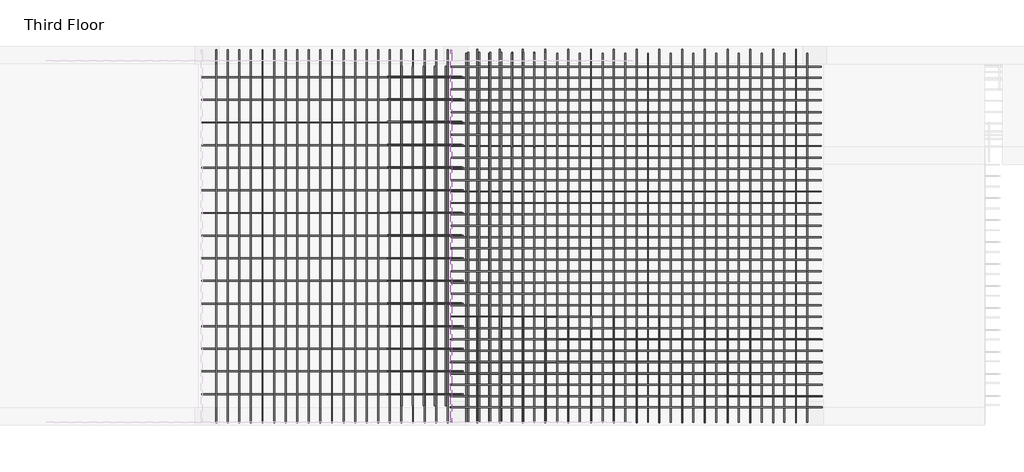
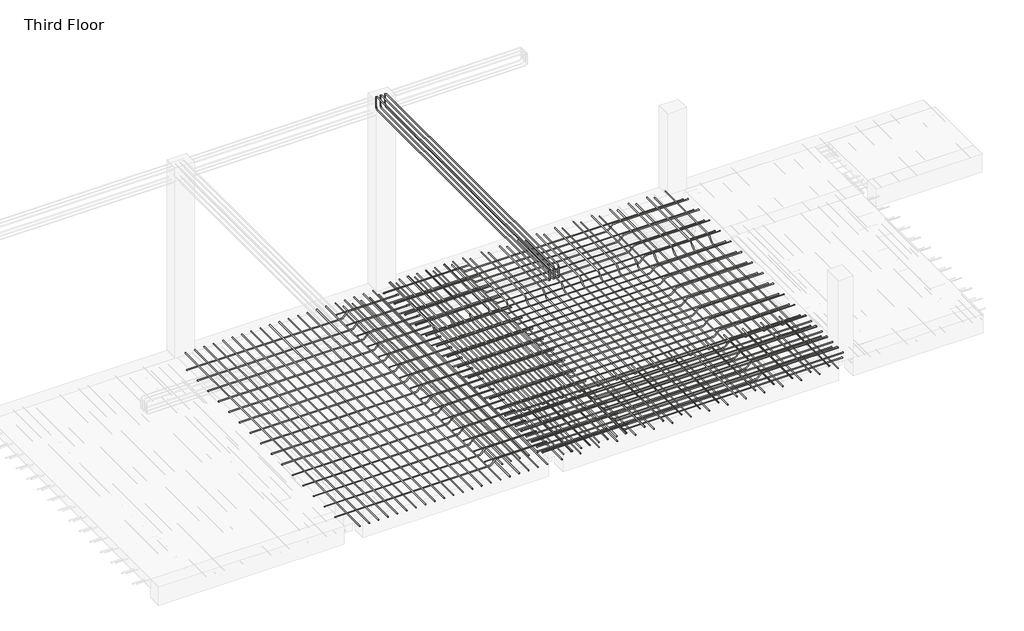
# One storey, part 3 of 4: 14 reinforcing bars.
"""IFC4 building model written with IfcOpenShell, lengths in millimetres."""

from ifc_helpers import new_model, si_unit, point, frame, origin, place, context, project, spatial, polyline, circle_curve, trimmed, segment, composite_curve, source, transform, mapped, element, save
from ifc_brep_helpers import swept_disk

model = new_model("IFC4")

# Units and contexts
model_context = context("Model", 3, world=origin())
ifc_project = project(units=[si_unit("LENGTHUNIT", "METRE", prefix="MILLI")], contexts=[model_context])

# Site, building, storey
site = spatial("IfcSite", under=ifc_project)
building = spatial("IfcBuilding", under=site)
storey = spatial("IfcBuildingStorey", under=building, Name="Third Floor", Elevation=9601.2)

# Reinforcing bars
placement = place(None, origin())
reinforcing_bar_shape = source(origin(), model_context, "Body", "SolidModel", [
    swept_disk(composite_curve([segment(polyline([(-2909.6112474, 5017.2334631, 12564.4994949), (-2909.6112474, 5017.2334631, 12712.4994949)]), True, "CONTINUOUS"), segment(trimmed(circle_curve(frame((-2909.6112474, 4971.2334631, 12712.4994949), z_axis=(1.0, 0.0, 0.0), x_axis=(0.0, 46.0, 0.0)), 46.0), [point((-2909.6112474, 5017.2334631, 12712.4994949))], [point((-2909.6112474, 4971.2334631, 12758.4994949))], True, "CARTESIAN"), True, "CONTINUOUS"), segment(polyline([(-2909.6112474, 4971.2334631, 12758.4994949), (-2909.6112474, 278.4334631, 12758.4994949)]), True, "CONTINUOUS"), segment(trimmed(circle_curve(frame((-2909.6112474, 278.4334631, 12712.4994949), z_axis=(1.0, 0.0, 0.0), x_axis=(0.0, 0.0, 46.0)), 46.0), [point((-2909.6112474, 278.4334631, 12758.4994949))], [point((-2909.6112474, 232.4334631, 12712.4994949))], True, "CARTESIAN"), True, "CONTINUOUS"), segment(polyline([(-2909.6112474, 232.4334631, 12712.4994949), (-2909.6112474, 232.4334631, 12564.4994949)]), True, "CONTINUOUS")], self_intersect=False), 6.0),
])
element("IfcReinforcingBar", 1, at=placement, inside=storey, context=model_context, shape_type="MappedRepresentation", body=[
    mapped(reinforcing_bar_shape, transform((0.0, 0.0, 0.0), x_axis=(1.0, 0.0, 0.0), y_axis=(0.0, 1.0, 0.0), z_axis=(0.0, 0.0, 1.0))),
    mapped(reinforcing_bar_shape, transform((71.1994949, 0.0, 0.0), x_axis=(1.0, 0.0, 0.0), y_axis=(0.0, 1.0, 0.0), z_axis=(0.0, 0.0, 1.0))),
    mapped(reinforcing_bar_shape, transform((142.3989899, 0.0, 0.0), x_axis=(1.0, 0.0, 0.0), y_axis=(0.0, 1.0, 0.0), z_axis=(0.0, 0.0, 1.0))),
])
reinforcing_bar_2_shape = source(origin(), model_context, "Body", "SolidModel", [
    swept_disk(composite_curve([segment(polyline([(-2909.6112474, 5017.2334631, 12733.9005051), (-2909.6112474, 5017.2334631, 12585.9005051)]), True, "CONTINUOUS"), segment(trimmed(circle_curve(frame((-2909.6112474, 4971.2334631, 12585.9005051), z_axis=(-1.0, 0.0, 0.0), x_axis=(0.0, 46.0, 0.0)), 46.0), [point((-2909.6112474, 5017.2334631, 12585.9005051))], [point((-2909.6112474, 4971.2334631, 12539.9005051))], True, "CARTESIAN"), True, "CONTINUOUS"), segment(polyline([(-2909.6112474, 4971.2334631, 12539.9005051), (-2909.6112474, 278.4334631, 12539.9005051)]), True, "CONTINUOUS"), segment(trimmed(circle_curve(frame((-2909.6112474, 278.4334631, 12585.9005051), z_axis=(-1.0, 0.0, 0.0), x_axis=(0.0, 0.0, -46.0)), 46.0), [point((-2909.6112474, 278.4334631, 12539.9005051))], [point((-2909.6112474, 232.4334631, 12585.9005051))], True, "CARTESIAN"), True, "CONTINUOUS"), segment(polyline([(-2909.6112474, 232.4334631, 12585.9005051), (-2909.6112474, 232.4334631, 12733.9005051)]), True, "CONTINUOUS")], self_intersect=False), 6.0),
])
element("IfcReinforcingBar", 2, at=placement, inside=storey, context=model_context, shape_type="MappedRepresentation", body=[
    mapped(reinforcing_bar_2_shape, transform((0.0, 0.0, 0.0), x_axis=(1.0, 0.0, 0.0), y_axis=(0.0, 1.0, 0.0), z_axis=(0.0, 0.0, 1.0))),
    mapped(reinforcing_bar_2_shape, transform((71.1994949, 0.0, 0.0), x_axis=(1.0, 0.0, 0.0), y_axis=(0.0, 1.0, 0.0), z_axis=(0.0, 0.0, 1.0))),
    mapped(reinforcing_bar_2_shape, transform((142.3989899, 0.0, 0.0), x_axis=(1.0, 0.0, 0.0), y_axis=(0.0, 1.0, 0.0), z_axis=(0.0, 0.0, 1.0))),
])
reinforcing_bar_3_shape = source(origin(), model_context, "Body", "SolidModel", [
    swept_disk(composite_curve([segment(polyline([(-2755.5109354, 590.4513536, 9570.2), (-3537.444222, 590.4513536, 9570.2)]), True, "CONTINUOUS"), segment(trimmed(circle_curve(frame((-3537.444222, 590.4513536, 9524.2), z_axis=(0.0, -1.0, 0.0), x_axis=(0.0, 0.0, 46.0)), 46.0), [point((-3537.444222, 590.4513536, 9570.2))], [point((-3569.9711339, 590.4513536, 9556.7269119))], True, "CARTESIAN"), True, "CONTINUOUS"), segment(polyline([(-3569.9711339, 590.4513536, 9556.7269119), (-3633.4249578, 590.4513536, 9493.2730881)]), True, "CONTINUOUS"), segment(trimmed(circle_curve(frame((-3665.9518697, 590.4513536, 9525.8), z_axis=(0.0, 1.0000000000000002, 0.0), x_axis=(32.52691189999996, 0.0, -32.526911899998595)), 46.0), [point((-3633.4249578, 590.4513536, 9493.2730881))], [point((-3665.9518697, 590.4513536, 9479.8))], True, "CARTESIAN"), True, "CONTINUOUS"), segment(polyline([(-3665.9518697, 590.4513536, 9479.8), (-6120.96376, 590.4513536, 9479.8)]), True, "CONTINUOUS")], self_intersect=False), 6.0),
])
element("IfcReinforcingBar", 3, at=placement, inside=storey, context=model_context, shape_type="MappedRepresentation", body=[
    mapped(reinforcing_bar_3_shape, transform((0.0, 0.0, 0.0), x_axis=(1.0, 0.0, 0.0), y_axis=(0.0, 1.0, 0.0), z_axis=(0.0, 0.0, 1.0))),
    mapped(reinforcing_bar_3_shape, transform((0.0, 291.2629007, 0.0), x_axis=(1.0, 0.0, 0.0), y_axis=(0.0, 1.0, 0.0), z_axis=(0.0, 0.0, 1.0))),
    mapped(reinforcing_bar_3_shape, transform((0.0, 582.5258014, 0.0), x_axis=(1.0, 0.0, 0.0), y_axis=(0.0, 1.0, 0.0), z_axis=(0.0, 0.0, 1.0))),
    mapped(reinforcing_bar_3_shape, transform((0.0, 873.7887021, 0.0), x_axis=(1.0, 0.0, 0.0), y_axis=(0.0, 1.0, 0.0), z_axis=(0.0, 0.0, 1.0))),
    mapped(reinforcing_bar_3_shape, transform((0.0, 1165.0516028, 0.0), x_axis=(1.0, 0.0, 0.0), y_axis=(0.0, 1.0, 0.0), z_axis=(0.0, 0.0, 1.0))),
    mapped(reinforcing_bar_3_shape, transform((0.0, 1456.3145035, 0.0), x_axis=(1.0, 0.0, 0.0), y_axis=(0.0, 1.0, 0.0), z_axis=(0.0, 0.0, 1.0))),
    mapped(reinforcing_bar_3_shape, transform((0.0, 1747.5774042, 0.0), x_axis=(1.0, 0.0, 0.0), y_axis=(0.0, 1.0, 0.0), z_axis=(0.0, 0.0, 1.0))),
    mapped(reinforcing_bar_3_shape, transform((0.0, 2038.8403049, 0.0), x_axis=(1.0, 0.0, 0.0), y_axis=(0.0, 1.0, 0.0), z_axis=(0.0, 0.0, 1.0))),
    mapped(reinforcing_bar_3_shape, transform((0.0, 2330.1032056, 0.0), x_axis=(1.0, 0.0, 0.0), y_axis=(0.0, 1.0, 0.0), z_axis=(0.0, 0.0, 1.0))),
    mapped(reinforcing_bar_3_shape, transform((0.0, 2621.3661063, 0.0), x_axis=(1.0, 0.0, 0.0), y_axis=(0.0, 1.0, 0.0), z_axis=(0.0, 0.0, 1.0))),
    mapped(reinforcing_bar_3_shape, transform((0.0, 2912.629007, 0.0), x_axis=(1.0, 0.0, 0.0), y_axis=(0.0, 1.0, 0.0), z_axis=(0.0, 0.0, 1.0))),
    mapped(reinforcing_bar_3_shape, transform((0.0, 3203.8919077, 0.0), x_axis=(1.0, 0.0, 0.0), y_axis=(0.0, 1.0, 0.0), z_axis=(0.0, 0.0, 1.0))),
    mapped(reinforcing_bar_3_shape, transform((0.0, 3495.1548084, 0.0), x_axis=(1.0, 0.0, 0.0), y_axis=(0.0, 1.0, 0.0), z_axis=(0.0, 0.0, 1.0))),
    mapped(reinforcing_bar_3_shape, transform((0.0, 3786.4177091, 0.0), x_axis=(1.0, 0.0, 0.0), y_axis=(0.0, 1.0, 0.0), z_axis=(0.0, 0.0, 1.0))),
    mapped(reinforcing_bar_3_shape, transform((0.0, 4077.6806098, 0.0), x_axis=(1.0, 0.0, 0.0), y_axis=(0.0, 1.0, 0.0), z_axis=(0.0, 0.0, 1.0))),
])
reinforcing_bar_4_shape = source(origin(), model_context, "Body", "SolidModel", [
    swept_disk(composite_curve([segment(polyline([(-3546.4250876, 4809.6334631, 9559.9006995), (-3546.4250876, 440.0334631, 9559.9006995)]), True, "CONTINUOUS")], self_intersect=False), 6.0),
])
element("IfcReinforcingBar", 4, at=placement, inside=storey, context=model_context, shape_type="MappedRepresentation", body=[
    mapped(reinforcing_bar_4_shape, transform((0.0, 0.0, 0.0), x_axis=(1.0, 0.0, 0.0), y_axis=(0.0, 1.0, 0.0), z_axis=(0.0, 0.0, 1.0))),
    mapped(reinforcing_bar_4_shape, transform((140.6783338, 0.0, 0.0), x_axis=(1.0, 0.0, 0.0), y_axis=(0.0, 1.0, 0.0), z_axis=(0.0, 0.0, 1.0))),
    mapped(reinforcing_bar_4_shape, transform((281.3566676, 0.0, 0.0), x_axis=(1.0, 0.0, 0.0), y_axis=(0.0, 1.0, 0.0), z_axis=(0.0, 0.0, 1.0))),
    mapped(reinforcing_bar_4_shape, transform((422.0350014, 0.0, 0.0), x_axis=(1.0, 0.0, 0.0), y_axis=(0.0, 1.0, 0.0), z_axis=(0.0, 0.0, 1.0))),
    mapped(reinforcing_bar_4_shape, transform((562.7133352, 0.0, 0.0), x_axis=(1.0, 0.0, 0.0), y_axis=(0.0, 1.0, 0.0), z_axis=(0.0, 0.0, 1.0))),
])
reinforcing_bar_5_shape = source(origin(), model_context, "Body", "SolidModel", [
    swept_disk(composite_curve([segment(polyline([(-2778.2123639, 4678.4115375, 9572.2), (-3737.2865297, 4678.4115375, 9572.2)]), True, "CONTINUOUS")], self_intersect=False), 4.0),
])
element("IfcReinforcingBar", 5, at=placement, inside=storey, context=model_context, shape_type="MappedRepresentation", body=[
    mapped(reinforcing_bar_5_shape, transform((0.0, 0.0, 0.0), x_axis=(1.0, 0.0, 0.0), y_axis=(0.0, 1.0, 0.0), z_axis=(0.0, 0.0, 1.0))),
    mapped(reinforcing_bar_5_shape, transform((0.0, -291.8025106, 0.0), x_axis=(1.0, 0.0, 0.0), y_axis=(0.0, 1.0, 0.0), z_axis=(0.0, 0.0, 1.0))),
    mapped(reinforcing_bar_5_shape, transform((0.0, -583.6050212, 0.0), x_axis=(1.0, 0.0, 0.0), y_axis=(0.0, 1.0, 0.0), z_axis=(0.0, 0.0, 1.0))),
    mapped(reinforcing_bar_5_shape, transform((0.0, -875.4075319, 0.0), x_axis=(1.0, 0.0, 0.0), y_axis=(0.0, 1.0, 0.0), z_axis=(0.0, 0.0, 1.0))),
    mapped(reinforcing_bar_5_shape, transform((0.0, -1167.2100425, 0.0), x_axis=(1.0, 0.0, 0.0), y_axis=(0.0, 1.0, 0.0), z_axis=(0.0, 0.0, 1.0))),
    mapped(reinforcing_bar_5_shape, transform((0.0, -1459.0125531, 0.0), x_axis=(1.0, 0.0, 0.0), y_axis=(0.0, 1.0, 0.0), z_axis=(0.0, 0.0, 1.0))),
    mapped(reinforcing_bar_5_shape, transform((0.0, -1750.8150637, 0.0), x_axis=(1.0, 0.0, 0.0), y_axis=(0.0, 1.0, 0.0), z_axis=(0.0, 0.0, 1.0))),
    mapped(reinforcing_bar_5_shape, transform((0.0, -2042.6175743, 0.0), x_axis=(1.0, 0.0, 0.0), y_axis=(0.0, 1.0, 0.0), z_axis=(0.0, 0.0, 1.0))),
    mapped(reinforcing_bar_5_shape, transform((0.0, -2334.420085, 0.0), x_axis=(1.0, 0.0, 0.0), y_axis=(0.0, 1.0, 0.0), z_axis=(0.0, 0.0, 1.0))),
    mapped(reinforcing_bar_5_shape, transform((0.0, -2626.2225956, 0.0), x_axis=(1.0, 0.0, 0.0), y_axis=(0.0, 1.0, 0.0), z_axis=(0.0, 0.0, 1.0))),
    mapped(reinforcing_bar_5_shape, transform((0.0, -2918.0251062, 0.0), x_axis=(1.0, 0.0, 0.0), y_axis=(0.0, 1.0, 0.0), z_axis=(0.0, 0.0, 1.0))),
    mapped(reinforcing_bar_5_shape, transform((0.0, -3209.8276168, 0.0), x_axis=(1.0, 0.0, 0.0), y_axis=(0.0, 1.0, 0.0), z_axis=(0.0, 0.0, 1.0))),
    mapped(reinforcing_bar_5_shape, transform((0.0, -3501.6301274, 0.0), x_axis=(1.0, 0.0, 0.0), y_axis=(0.0, 1.0, 0.0), z_axis=(0.0, 0.0, 1.0))),
    mapped(reinforcing_bar_5_shape, transform((0.0, -3793.4326381, 0.0), x_axis=(1.0, 0.0, 0.0), y_axis=(0.0, 1.0, 0.0), z_axis=(0.0, 0.0, 1.0))),
    mapped(reinforcing_bar_5_shape, transform((0.0, -4085.2351487, 0.0), x_axis=(1.0, 0.0, 0.0), y_axis=(0.0, 1.0, 0.0), z_axis=(0.0, 0.0, 1.0))),
])
reinforcing_bar_6_shape = source(origin(), model_context, "Body", "SolidModel", [
    swept_disk(composite_curve([segment(polyline([(-2956.7117524, 218.9117605, 9488.3387401), (-2956.7117524, 5019.9992064, 9488.3387401)]), True, "CONTINUOUS")], self_intersect=False), 6.0),
])
element("IfcReinforcingBar", 6, at=placement, inside=storey, context=model_context, shape_type="MappedRepresentation", body=[
    mapped(reinforcing_bar_6_shape, transform((0.0, 0.0, 0.0), x_axis=(1.0, 0.0, 0.0), y_axis=(0.0, 1.0, 0.0), z_axis=(0.0, 0.0, 1.0))),
    mapped(reinforcing_bar_6_shape, transform((-149.025, 0.0, 0.0), x_axis=(1.0, 0.0, 0.0), y_axis=(0.0, 1.0, 0.0), z_axis=(0.0, 0.0, 1.0))),
    mapped(reinforcing_bar_6_shape, transform((-298.05, 0.0, 0.0), x_axis=(1.0, 0.0, 0.0), y_axis=(0.0, 1.0, 0.0), z_axis=(0.0, 0.0, 1.0))),
    mapped(reinforcing_bar_6_shape, transform((-447.075, 0.0, 0.0), x_axis=(1.0, 0.0, 0.0), y_axis=(0.0, 1.0, 0.0), z_axis=(0.0, 0.0, 1.0))),
    mapped(reinforcing_bar_6_shape, transform((-596.1, 0.0, 0.0), x_axis=(1.0, 0.0, 0.0), y_axis=(0.0, 1.0, 0.0), z_axis=(0.0, 0.0, 1.0))),
    mapped(reinforcing_bar_6_shape, transform((-745.125, 0.0, 0.0), x_axis=(1.0, 0.0, 0.0), y_axis=(0.0, 1.0, 0.0), z_axis=(0.0, 0.0, 1.0))),
    mapped(reinforcing_bar_6_shape, transform((-894.15, 0.0, 0.0), x_axis=(1.0, 0.0, 0.0), y_axis=(0.0, 1.0, 0.0), z_axis=(0.0, 0.0, 1.0))),
    mapped(reinforcing_bar_6_shape, transform((-1043.175, 0.0, 0.0), x_axis=(1.0, 0.0, 0.0), y_axis=(0.0, 1.0, 0.0), z_axis=(0.0, 0.0, 1.0))),
    mapped(reinforcing_bar_6_shape, transform((-1192.2, 0.0, 0.0), x_axis=(1.0, 0.0, 0.0), y_axis=(0.0, 1.0, 0.0), z_axis=(0.0, 0.0, 1.0))),
    mapped(reinforcing_bar_6_shape, transform((-1341.225, 0.0, 0.0), x_axis=(1.0, 0.0, 0.0), y_axis=(0.0, 1.0, 0.0), z_axis=(0.0, 0.0, 1.0))),
    mapped(reinforcing_bar_6_shape, transform((-1490.25, 0.0, 0.0), x_axis=(1.0, 0.0, 0.0), y_axis=(0.0, 1.0, 0.0), z_axis=(0.0, 0.0, 1.0))),
    mapped(reinforcing_bar_6_shape, transform((-1639.275, 0.0, 0.0), x_axis=(1.0, 0.0, 0.0), y_axis=(0.0, 1.0, 0.0), z_axis=(0.0, 0.0, 1.0))),
    mapped(reinforcing_bar_6_shape, transform((-1788.3, 0.0, 0.0), x_axis=(1.0, 0.0, 0.0), y_axis=(0.0, 1.0, 0.0), z_axis=(0.0, 0.0, 1.0))),
    mapped(reinforcing_bar_6_shape, transform((-1937.325, 0.0, 0.0), x_axis=(1.0, 0.0, 0.0), y_axis=(0.0, 1.0, 0.0), z_axis=(0.0, 0.0, 1.0))),
    mapped(reinforcing_bar_6_shape, transform((-2086.35, 0.0, 0.0), x_axis=(1.0, 0.0, 0.0), y_axis=(0.0, 1.0, 0.0), z_axis=(0.0, 0.0, 1.0))),
    mapped(reinforcing_bar_6_shape, transform((-2235.375, 0.0, 0.0), x_axis=(1.0, 0.0, 0.0), y_axis=(0.0, 1.0, 0.0), z_axis=(0.0, 0.0, 1.0))),
    mapped(reinforcing_bar_6_shape, transform((-2384.4, 0.0, 0.0), x_axis=(1.0, 0.0, 0.0), y_axis=(0.0, 1.0, 0.0), z_axis=(0.0, 0.0, 1.0))),
    mapped(reinforcing_bar_6_shape, transform((-2533.425, 0.0, 0.0), x_axis=(1.0, 0.0, 0.0), y_axis=(0.0, 1.0, 0.0), z_axis=(0.0, 0.0, 1.0))),
    mapped(reinforcing_bar_6_shape, transform((-2682.45, 0.0, 0.0), x_axis=(1.0, 0.0, 0.0), y_axis=(0.0, 1.0, 0.0), z_axis=(0.0, 0.0, 1.0))),
    mapped(reinforcing_bar_6_shape, transform((-2831.475, 0.0, 0.0), x_axis=(1.0, 0.0, 0.0), y_axis=(0.0, 1.0, 0.0), z_axis=(0.0, 0.0, 1.0))),
    mapped(reinforcing_bar_6_shape, transform((-2980.5, 0.0, 0.0), x_axis=(1.0, 0.0, 0.0), y_axis=(0.0, 1.0, 0.0), z_axis=(0.0, 0.0, 1.0))),
])
reinforcing_bar_7_shape = source(origin(), model_context, "Body", "SolidModel", [
    swept_disk(composite_curve([segment(polyline([(-1702.6950858, 4992.3164819, 9554.9006995), (-1702.6950858, 234.3272052, 9554.9006995)]), True, "CONTINUOUS")], self_intersect=False), 6.0),
])
element("IfcReinforcingBar", 7, at=placement, inside=storey, context=model_context, shape_type="MappedRepresentation", body=[
    mapped(reinforcing_bar_7_shape, transform((0.0, 0.0, 0.0), x_axis=(1.0, 0.0, 0.0), y_axis=(0.0, 1.0, 0.0), z_axis=(0.0, 0.0, 1.0))),
    mapped(reinforcing_bar_7_shape, transform((-141.4880952, 0.0, 0.0), x_axis=(1.0, 0.0, 0.0), y_axis=(0.0, 1.0, 0.0), z_axis=(0.0, 0.0, 1.0))),
    mapped(reinforcing_bar_7_shape, transform((-282.9761905, 0.0, 0.0), x_axis=(1.0, 0.0, 0.0), y_axis=(0.0, 1.0, 0.0), z_axis=(0.0, 0.0, 1.0))),
    mapped(reinforcing_bar_7_shape, transform((-424.4642857, 0.0, 0.0), x_axis=(1.0, 0.0, 0.0), y_axis=(0.0, 1.0, 0.0), z_axis=(0.0, 0.0, 1.0))),
    mapped(reinforcing_bar_7_shape, transform((-565.952381, 0.0, 0.0), x_axis=(1.0, 0.0, 0.0), y_axis=(0.0, 1.0, 0.0), z_axis=(0.0, 0.0, 1.0))),
    mapped(reinforcing_bar_7_shape, transform((-707.4404762, 0.0, 0.0), x_axis=(1.0, 0.0, 0.0), y_axis=(0.0, 1.0, 0.0), z_axis=(0.0, 0.0, 1.0))),
    mapped(reinforcing_bar_7_shape, transform((-848.9285714, 0.0, 0.0), x_axis=(1.0, 0.0, 0.0), y_axis=(0.0, 1.0, 0.0), z_axis=(0.0, 0.0, 1.0))),
    mapped(reinforcing_bar_7_shape, transform((-990.4166667, 0.0, 0.0), x_axis=(1.0, 0.0, 0.0), y_axis=(0.0, 1.0, 0.0), z_axis=(0.0, 0.0, 1.0))),
])
reinforcing_bar_8_shape = source(origin(), model_context, "Body", "SolidModel", [
    swept_disk(composite_curve([segment(polyline([(-2905.905155, 4803.6334631, 9567.1687876), (-1727.9771661, 4803.6334631, 9567.1687876)]), True, "CONTINUOUS"), segment(trimmed(circle_curve(frame((-1727.9771661, 4803.6334631, 9521.1687876), z_axis=(0.0, 1.0, 0.0), x_axis=(0.0, 0.0, 46.0)), 46.0), [point((-1727.9771661, 4803.6334631, 9567.1687876))], [point((-1695.4502541, 4803.6334631, 9553.6956996))], True, "CARTESIAN"), True, "CONTINUOUS"), segment(polyline([(-1695.4502541, 4803.6334631, 9553.6956996), (-1634.9899166, 4803.6334631, 9493.2353621)]), True, "CONTINUOUS"), segment(trimmed(circle_curve(frame((-1602.4630047, 4803.6334631, 9525.762274), z_axis=(0.0, -1.0, 0.0), x_axis=(-32.52691189999996, 0.0, -32.526911900000414)), 46.0), [point((-1634.9899166, 4803.6334631, 9493.2353621))], [point((-1602.4630047, 4803.6334631, 9479.762274))], True, "CARTESIAN"), True, "CONTINUOUS"), segment(polyline([(-1602.4630047, 4803.6334631, 9479.762274), (1847.5013288, 4803.6334631, 9479.762274)]), True, "CONTINUOUS")], self_intersect=False), 6.0),
])
element("IfcReinforcingBar", 8, at=placement, inside=storey, context=model_context, shape_type="MappedRepresentation", body=[
    mapped(reinforcing_bar_8_shape, transform((0.0, 0.0, 0.0), x_axis=(1.0, 0.0, 0.0), y_axis=(0.0, 1.0, 0.0), z_axis=(0.0, 0.0, 1.0))),
    mapped(reinforcing_bar_8_shape, transform((0.0, -292.3066667, 0.0), x_axis=(1.0, 0.0, 0.0), y_axis=(0.0, 1.0, 0.0), z_axis=(0.0, 0.0, 1.0))),
    mapped(reinforcing_bar_8_shape, transform((0.0, -584.6133333, 0.0), x_axis=(1.0, 0.0, 0.0), y_axis=(0.0, 1.0, 0.0), z_axis=(0.0, 0.0, 1.0))),
    mapped(reinforcing_bar_8_shape, transform((0.0, -876.92, 0.0), x_axis=(1.0, 0.0, 0.0), y_axis=(0.0, 1.0, 0.0), z_axis=(0.0, 0.0, 1.0))),
    mapped(reinforcing_bar_8_shape, transform((0.0, -1169.2266667, 0.0), x_axis=(1.0, 0.0, 0.0), y_axis=(0.0, 1.0, 0.0), z_axis=(0.0, 0.0, 1.0))),
    mapped(reinforcing_bar_8_shape, transform((0.0, -1461.5333333, 0.0), x_axis=(1.0, 0.0, 0.0), y_axis=(0.0, 1.0, 0.0), z_axis=(0.0, 0.0, 1.0))),
    mapped(reinforcing_bar_8_shape, transform((0.0, -1753.84, 0.0), x_axis=(1.0, 0.0, 0.0), y_axis=(0.0, 1.0, 0.0), z_axis=(0.0, 0.0, 1.0))),
    mapped(reinforcing_bar_8_shape, transform((0.0, -2046.1466667, 0.0), x_axis=(1.0, 0.0, 0.0), y_axis=(0.0, 1.0, 0.0), z_axis=(0.0, 0.0, 1.0))),
    mapped(reinforcing_bar_8_shape, transform((0.0, -2338.4533333, 0.0), x_axis=(1.0, 0.0, 0.0), y_axis=(0.0, 1.0, 0.0), z_axis=(0.0, 0.0, 1.0))),
    mapped(reinforcing_bar_8_shape, transform((0.0, -2630.76, 0.0), x_axis=(1.0, 0.0, 0.0), y_axis=(0.0, 1.0, 0.0), z_axis=(0.0, 0.0, 1.0))),
    mapped(reinforcing_bar_8_shape, transform((0.0, -2923.0666667, 0.0), x_axis=(1.0, 0.0, 0.0), y_axis=(0.0, 1.0, 0.0), z_axis=(0.0, 0.0, 1.0))),
    mapped(reinforcing_bar_8_shape, transform((0.0, -3215.3733333, 0.0), x_axis=(1.0, 0.0, 0.0), y_axis=(0.0, 1.0, 0.0), z_axis=(0.0, 0.0, 1.0))),
    mapped(reinforcing_bar_8_shape, transform((0.0, -3507.68, 0.0), x_axis=(1.0, 0.0, 0.0), y_axis=(0.0, 1.0, 0.0), z_axis=(0.0, 0.0, 1.0))),
    mapped(reinforcing_bar_8_shape, transform((0.0, -3799.9866667, 0.0), x_axis=(1.0, 0.0, 0.0), y_axis=(0.0, 1.0, 0.0), z_axis=(0.0, 0.0, 1.0))),
    mapped(reinforcing_bar_8_shape, transform((0.0, -4092.2933333, 0.0), x_axis=(1.0, 0.0, 0.0), y_axis=(0.0, 1.0, 0.0), z_axis=(0.0, 0.0, 1.0))),
    mapped(reinforcing_bar_8_shape, transform((0.0, -4384.6, 0.0), x_axis=(1.0, 0.0, 0.0), y_axis=(0.0, 1.0, 0.0), z_axis=(0.0, 0.0, 1.0))),
])
reinforcing_bar_9_shape = source(origin(), model_context, "Body", "SolidModel", [
    swept_disk(composite_curve([segment(polyline([(-2911.6309684, 4803.6334631, 9564.6017937), (-1557.9199073, 4803.6334631, 9564.6017937)]), True, "CONTINUOUS")], self_intersect=False), 6.0),
])
element("IfcReinforcingBar", 9, at=placement, inside=storey, context=model_context, shape_type="MappedRepresentation", body=[
    mapped(reinforcing_bar_9_shape, transform((0.0, 0.0, 0.0), x_axis=(1.0, 0.0, 0.0), y_axis=(0.0, 1.0, 0.0), z_axis=(0.0, 0.0, 1.0))),
    mapped(reinforcing_bar_9_shape, transform((0.0, -292.3066667, 0.0), x_axis=(1.0, 0.0, 0.0), y_axis=(0.0, 1.0, 0.0), z_axis=(0.0, 0.0, 1.0))),
    mapped(reinforcing_bar_9_shape, transform((0.0, -584.6133333, 0.0), x_axis=(1.0, 0.0, 0.0), y_axis=(0.0, 1.0, 0.0), z_axis=(0.0, 0.0, 1.0))),
    mapped(reinforcing_bar_9_shape, transform((0.0, -876.92, 0.0), x_axis=(1.0, 0.0, 0.0), y_axis=(0.0, 1.0, 0.0), z_axis=(0.0, 0.0, 1.0))),
    mapped(reinforcing_bar_9_shape, transform((0.0, -1169.2266667, 0.0), x_axis=(1.0, 0.0, 0.0), y_axis=(0.0, 1.0, 0.0), z_axis=(0.0, 0.0, 1.0))),
    mapped(reinforcing_bar_9_shape, transform((0.0, -1461.5333333, 0.0), x_axis=(1.0, 0.0, 0.0), y_axis=(0.0, 1.0, 0.0), z_axis=(0.0, 0.0, 1.0))),
    mapped(reinforcing_bar_9_shape, transform((0.0, -1753.84, 0.0), x_axis=(1.0, 0.0, 0.0), y_axis=(0.0, 1.0, 0.0), z_axis=(0.0, 0.0, 1.0))),
    mapped(reinforcing_bar_9_shape, transform((0.0, -2046.1466667, 0.0), x_axis=(1.0, 0.0, 0.0), y_axis=(0.0, 1.0, 0.0), z_axis=(0.0, 0.0, 1.0))),
    mapped(reinforcing_bar_9_shape, transform((0.0, -2338.4533333, 0.0), x_axis=(1.0, 0.0, 0.0), y_axis=(0.0, 1.0, 0.0), z_axis=(0.0, 0.0, 1.0))),
    mapped(reinforcing_bar_9_shape, transform((0.0, -2630.76, 0.0), x_axis=(1.0, 0.0, 0.0), y_axis=(0.0, 1.0, 0.0), z_axis=(0.0, 0.0, 1.0))),
    mapped(reinforcing_bar_9_shape, transform((0.0, -2923.0666667, 0.0), x_axis=(1.0, 0.0, 0.0), y_axis=(0.0, 1.0, 0.0), z_axis=(0.0, 0.0, 1.0))),
    mapped(reinforcing_bar_9_shape, transform((0.0, -3215.3733333, 0.0), x_axis=(1.0, 0.0, 0.0), y_axis=(0.0, 1.0, 0.0), z_axis=(0.0, 0.0, 1.0))),
    mapped(reinforcing_bar_9_shape, transform((0.0, -3507.68, 0.0), x_axis=(1.0, 0.0, 0.0), y_axis=(0.0, 1.0, 0.0), z_axis=(0.0, 0.0, 1.0))),
    mapped(reinforcing_bar_9_shape, transform((0.0, -3799.9866667, 0.0), x_axis=(1.0, 0.0, 0.0), y_axis=(0.0, 1.0, 0.0), z_axis=(0.0, 0.0, 1.0))),
    mapped(reinforcing_bar_9_shape, transform((0.0, -4092.2933333, 0.0), x_axis=(1.0, 0.0, 0.0), y_axis=(0.0, 1.0, 0.0), z_axis=(0.0, 0.0, 1.0))),
    mapped(reinforcing_bar_9_shape, transform((0.0, -4384.6, 0.0), x_axis=(1.0, 0.0, 0.0), y_axis=(0.0, 1.0, 0.0), z_axis=(0.0, 0.0, 1.0))),
])
reinforcing_bar_10_shape = source(origin(), model_context, "Body", "SolidModel", [
    swept_disk(composite_curve([segment(polyline([(1849.122149, 559.2793552, 9567.1687876), (670.8521547, 559.2793552, 9567.1687876)]), True, "CONTINUOUS"), segment(trimmed(circle_curve(frame((670.8521547, 559.2793552, 9521.1687876), z_axis=(0.0, -1.0, 0.0), x_axis=(0.0, 0.0, 46.0)), 46.0), [point((670.8521547, 559.2793552, 9567.1687876))], [point((638.3252427, 559.2793552, 9553.6956996))], True, "CARTESIAN"), True, "CONTINUOUS"), segment(polyline([(638.3252427, 559.2793552, 9553.6956996), (577.8649052, 559.2793552, 9493.2353621)]), True, "CONTINUOUS"), segment(trimmed(circle_curve(frame((545.3379933, 559.2793552, 9525.762274), z_axis=(0.0, 1.0000000000000002, 0.0), x_axis=(32.52691189999996, 0.0, -32.526911900000414)), 46.0), [point((577.8649052, 559.2793552, 9493.2353621))], [point((545.3379933, 559.2793552, 9479.762274))], True, "CARTESIAN"), True, "CONTINUOUS"), segment(polyline([(545.3379933, 559.2793552, 9479.762274), (-2914.2248337, 559.2793552, 9479.762274)]), True, "CONTINUOUS")], self_intersect=False), 6.0),
])
element("IfcReinforcingBar", 10, at=placement, inside=storey, context=model_context, shape_type="MappedRepresentation", body=[
    mapped(reinforcing_bar_10_shape, transform((0.0, 0.0, 0.0), x_axis=(1.0, 0.0, 0.0), y_axis=(0.0, 1.0, 0.0), z_axis=(0.0, 0.0, 1.0))),
    mapped(reinforcing_bar_10_shape, transform((0.0, 293.1320516, 0.0), x_axis=(1.0, 0.0, 0.0), y_axis=(0.0, 1.0, 0.0), z_axis=(0.0, 0.0, 1.0))),
    mapped(reinforcing_bar_10_shape, transform((0.0, 586.2641031, 0.0), x_axis=(1.0, 0.0, 0.0), y_axis=(0.0, 1.0, 0.0), z_axis=(0.0, 0.0, 1.0))),
    mapped(reinforcing_bar_10_shape, transform((0.0, 879.3961547, 0.0), x_axis=(1.0, 0.0, 0.0), y_axis=(0.0, 1.0, 0.0), z_axis=(0.0, 0.0, 1.0))),
    mapped(reinforcing_bar_10_shape, transform((0.0, 1172.5282063, 0.0), x_axis=(1.0, 0.0, 0.0), y_axis=(0.0, 1.0, 0.0), z_axis=(0.0, 0.0, 1.0))),
    mapped(reinforcing_bar_10_shape, transform((0.0, 1465.6602578, 0.0), x_axis=(1.0, 0.0, 0.0), y_axis=(0.0, 1.0, 0.0), z_axis=(0.0, 0.0, 1.0))),
    mapped(reinforcing_bar_10_shape, transform((0.0, 1758.7923094, 0.0), x_axis=(1.0, 0.0, 0.0), y_axis=(0.0, 1.0, 0.0), z_axis=(0.0, 0.0, 1.0))),
    mapped(reinforcing_bar_10_shape, transform((0.0, 2051.924361, 0.0), x_axis=(1.0, 0.0, 0.0), y_axis=(0.0, 1.0, 0.0), z_axis=(0.0, 0.0, 1.0))),
    mapped(reinforcing_bar_10_shape, transform((0.0, 2345.0564125, 0.0), x_axis=(1.0, 0.0, 0.0), y_axis=(0.0, 1.0, 0.0), z_axis=(0.0, 0.0, 1.0))),
    mapped(reinforcing_bar_10_shape, transform((0.0, 2638.1884641, 0.0), x_axis=(1.0, 0.0, 0.0), y_axis=(0.0, 1.0, 0.0), z_axis=(0.0, 0.0, 1.0))),
    mapped(reinforcing_bar_10_shape, transform((0.0, 2931.3205157, 0.0), x_axis=(1.0, 0.0, 0.0), y_axis=(0.0, 1.0, 0.0), z_axis=(0.0, 0.0, 1.0))),
    mapped(reinforcing_bar_10_shape, transform((0.0, 3224.4525672, 0.0), x_axis=(1.0, 0.0, 0.0), y_axis=(0.0, 1.0, 0.0), z_axis=(0.0, 0.0, 1.0))),
    mapped(reinforcing_bar_10_shape, transform((0.0, 3517.5846188, 0.0), x_axis=(1.0, 0.0, 0.0), y_axis=(0.0, 1.0, 0.0), z_axis=(0.0, 0.0, 1.0))),
    mapped(reinforcing_bar_10_shape, transform((0.0, 3810.7166704, 0.0), x_axis=(1.0, 0.0, 0.0), y_axis=(0.0, 1.0, 0.0), z_axis=(0.0, 0.0, 1.0))),
    mapped(reinforcing_bar_10_shape, transform((0.0, 4103.848722, 0.0), x_axis=(1.0, 0.0, 0.0), y_axis=(0.0, 1.0, 0.0), z_axis=(0.0, 0.0, 1.0))),
])
reinforcing_bar_11_shape = source(origin(), model_context, "Body", "SolidModel", [
    swept_disk(composite_curve([segment(polyline([(1667.8254733, 4978.61046, 9567.1687876), (1667.8254733, 3800.6824711, 9567.1687876)]), True, "CONTINUOUS"), segment(trimmed(circle_curve(frame((1667.8254733, 3800.6824711, 9521.1687876), z_axis=(1.0, 0.0, 0.0), x_axis=(0.0, 0.0, 46.0)), 46.0), [point((1667.8254733, 3800.6824711, 9567.1687876))], [point((1667.8254733, 3768.1555592, 9553.6956996))], True, "CARTESIAN"), True, "CONTINUOUS"), segment(polyline([(1667.8254733, 3768.1555592, 9553.6956996), (1667.8254733, 3707.6952216, 9493.2353621)]), True, "CONTINUOUS"), segment(trimmed(circle_curve(frame((1667.8254733, 3675.1683097, 9525.762274), z_axis=(-1.0, 0.0, 0.0), x_axis=(0.0, 32.52691189999996, -32.526911900000414)), 46.0), [point((1667.8254733, 3707.6952216, 9493.2353621))], [point((1667.8254733, 3675.1683097, 9479.762274))], True, "CARTESIAN"), True, "CONTINUOUS"), segment(polyline([(1667.8254733, 3675.1683097, 9479.762274), (1667.8254733, 225.2039762, 9479.762274)]), True, "CONTINUOUS")], self_intersect=False), 6.0),
])
element("IfcReinforcingBar", 11, at=placement, inside=storey, context=model_context, shape_type="MappedRepresentation", body=[
    mapped(reinforcing_bar_11_shape, transform((0.0, 0.0, 0.0), x_axis=(1.0, 0.0, 0.0), y_axis=(0.0, 1.0, 0.0), z_axis=(0.0, 0.0, 1.0))),
    mapped(reinforcing_bar_11_shape, transform((-292.44, 0.0, 0.0), x_axis=(1.0, 0.0, 0.0), y_axis=(0.0, 1.0, 0.0), z_axis=(0.0, 0.0, 1.0))),
    mapped(reinforcing_bar_11_shape, transform((-584.88, 0.0, 0.0), x_axis=(1.0, 0.0, 0.0), y_axis=(0.0, 1.0, 0.0), z_axis=(0.0, 0.0, 1.0))),
    mapped(reinforcing_bar_11_shape, transform((-877.32, 0.0, 0.0), x_axis=(1.0, 0.0, 0.0), y_axis=(0.0, 1.0, 0.0), z_axis=(0.0, 0.0, 1.0))),
    mapped(reinforcing_bar_11_shape, transform((-1169.76, 0.0, 0.0), x_axis=(1.0, 0.0, 0.0), y_axis=(0.0, 1.0, 0.0), z_axis=(0.0, 0.0, 1.0))),
    mapped(reinforcing_bar_11_shape, transform((-1462.2, 0.0, 0.0), x_axis=(1.0, 0.0, 0.0), y_axis=(0.0, 1.0, 0.0), z_axis=(0.0, 0.0, 1.0))),
    mapped(reinforcing_bar_11_shape, transform((-1754.64, 0.0, 0.0), x_axis=(1.0, 0.0, 0.0), y_axis=(0.0, 1.0, 0.0), z_axis=(0.0, 0.0, 1.0))),
    mapped(reinforcing_bar_11_shape, transform((-2047.08, 0.0, 0.0), x_axis=(1.0, 0.0, 0.0), y_axis=(0.0, 1.0, 0.0), z_axis=(0.0, 0.0, 1.0))),
    mapped(reinforcing_bar_11_shape, transform((-2339.52, 0.0, 0.0), x_axis=(1.0, 0.0, 0.0), y_axis=(0.0, 1.0, 0.0), z_axis=(0.0, 0.0, 1.0))),
    mapped(reinforcing_bar_11_shape, transform((-2631.96, 0.0, 0.0), x_axis=(1.0, 0.0, 0.0), y_axis=(0.0, 1.0, 0.0), z_axis=(0.0, 0.0, 1.0))),
    mapped(reinforcing_bar_11_shape, transform((-2924.4, 0.0, 0.0), x_axis=(1.0, 0.0, 0.0), y_axis=(0.0, 1.0, 0.0), z_axis=(0.0, 0.0, 1.0))),
    mapped(reinforcing_bar_11_shape, transform((-3216.84, 0.0, 0.0), x_axis=(1.0, 0.0, 0.0), y_axis=(0.0, 1.0, 0.0), z_axis=(0.0, 0.0, 1.0))),
    mapped(reinforcing_bar_11_shape, transform((-3509.28, 0.0, 0.0), x_axis=(1.0, 0.0, 0.0), y_axis=(0.0, 1.0, 0.0), z_axis=(0.0, 0.0, 1.0))),
    mapped(reinforcing_bar_11_shape, transform((-3801.72, 0.0, 0.0), x_axis=(1.0, 0.0, 0.0), y_axis=(0.0, 1.0, 0.0), z_axis=(0.0, 0.0, 1.0))),
    mapped(reinforcing_bar_11_shape, transform((-4094.16, 0.0, 0.0), x_axis=(1.0, 0.0, 0.0), y_axis=(0.0, 1.0, 0.0), z_axis=(0.0, 0.0, 1.0))),
    mapped(reinforcing_bar_11_shape, transform((-4386.6, 0.0, 0.0), x_axis=(1.0, 0.0, 0.0), y_axis=(0.0, 1.0, 0.0), z_axis=(0.0, 0.0, 1.0))),
])
reinforcing_bar_12_shape = source(origin(), model_context, "Body", "SolidModel", [
    swept_disk(composite_curve([segment(polyline([(1861.271842, 1438.6755099, 9555.2697281), (-2926.3745267, 1438.6755099, 9555.2697281)]), True, "CONTINUOUS")], self_intersect=False), 6.0),
])
element("IfcReinforcingBar", 12, at=placement, inside=storey, context=model_context, shape_type="MappedRepresentation", body=[
    mapped(reinforcing_bar_12_shape, transform((0.0, 0.0, 0.0), x_axis=(1.0, 0.0, 0.0), y_axis=(0.0, 1.0, 0.0), z_axis=(0.0, 0.0, 1.0))),
    mapped(reinforcing_bar_12_shape, transform((0.0, -145.6631495, 0.0), x_axis=(1.0, 0.0, 0.0), y_axis=(0.0, 1.0, 0.0), z_axis=(0.0, 0.0, 1.0))),
    mapped(reinforcing_bar_12_shape, transform((0.0, -291.3262991, 0.0), x_axis=(1.0, 0.0, 0.0), y_axis=(0.0, 1.0, 0.0), z_axis=(0.0, 0.0, 1.0))),
    mapped(reinforcing_bar_12_shape, transform((0.0, -436.9894486, 0.0), x_axis=(1.0, 0.0, 0.0), y_axis=(0.0, 1.0, 0.0), z_axis=(0.0, 0.0, 1.0))),
    mapped(reinforcing_bar_12_shape, transform((0.0, -582.6525982, 0.0), x_axis=(1.0, 0.0, 0.0), y_axis=(0.0, 1.0, 0.0), z_axis=(0.0, 0.0, 1.0))),
    mapped(reinforcing_bar_12_shape, transform((0.0, -728.3157477, 0.0), x_axis=(1.0, 0.0, 0.0), y_axis=(0.0, 1.0, 0.0), z_axis=(0.0, 0.0, 1.0))),
    mapped(reinforcing_bar_12_shape, transform((0.0, -873.9788973, 0.0), x_axis=(1.0, 0.0, 0.0), y_axis=(0.0, 1.0, 0.0), z_axis=(0.0, 0.0, 1.0))),
    mapped(reinforcing_bar_12_shape, transform((0.0, -1019.6420468, 0.0), x_axis=(1.0, 0.0, 0.0), y_axis=(0.0, 1.0, 0.0), z_axis=(0.0, 0.0, 1.0))),
])
reinforcing_bar_13_shape = source(origin(), model_context, "Body", "SolidModel", [
    swept_disk(composite_curve([segment(polyline([(-2578.5286346, 223.5831561, 9567.1687876), (-2578.5286346, 1401.8531503, 9567.1687876)]), True, "CONTINUOUS"), segment(trimmed(circle_curve(frame((-2578.5286346, 1401.8531503, 9521.1687876), z_axis=(-1.0, 0.0, 0.0), x_axis=(0.0, 0.0, 46.0)), 46.0), [point((-2578.5286346, 1401.8531503, 9567.1687876))], [point((-2578.5286346, 1434.3800623, 9553.6956996))], True, "CARTESIAN"), True, "CONTINUOUS"), segment(polyline([(-2578.5286346, 1434.3800623, 9553.6956996), (-2578.5286346, 1494.8026738, 9493.2730881)]), True, "CONTINUOUS"), segment(trimmed(circle_curve(frame((-2578.5286346, 1527.3295857, 9525.8), z_axis=(1.0, 0.0, 0.0), x_axis=(0.0, -32.52691189999996, -32.526911899998595)), 46.0), [point((-2578.5286346, 1494.8026738, 9493.2730881))], [point((-2578.5286346, 1527.3295857, 9479.8))], True, "CARTESIAN"), True, "CONTINUOUS"), segment(polyline([(-2578.5286346, 1527.3295857, 9479.8), (-2578.5286346, 5025.6536732, 9479.8)]), True, "CONTINUOUS")], self_intersect=False), 6.0),
])
element("IfcReinforcingBar", 13, at=placement, inside=storey, context=model_context, shape_type="MappedRepresentation", body=[
    mapped(reinforcing_bar_13_shape, transform((0.0, 0.0, 0.0), x_axis=(1.0, 0.0, 0.0), y_axis=(0.0, 1.0, 0.0), z_axis=(0.0, 0.0, 1.0))),
    mapped(reinforcing_bar_13_shape, transform((293.1320516, 0.0, 0.0), x_axis=(1.0, 0.0, 0.0), y_axis=(0.0, 1.0, 0.0), z_axis=(0.0, 0.0, 1.0))),
    mapped(reinforcing_bar_13_shape, transform((586.2641031, 0.0, 0.0), x_axis=(1.0, 0.0, 0.0), y_axis=(0.0, 1.0, 0.0), z_axis=(0.0, 0.0, 1.0))),
    mapped(reinforcing_bar_13_shape, transform((879.3961547, 0.0, 0.0), x_axis=(1.0, 0.0, 0.0), y_axis=(0.0, 1.0, 0.0), z_axis=(0.0, 0.0, 1.0))),
    mapped(reinforcing_bar_13_shape, transform((1172.5282063, 0.0, 0.0), x_axis=(1.0, 0.0, 0.0), y_axis=(0.0, 1.0, 0.0), z_axis=(0.0, 0.0, 1.0))),
    mapped(reinforcing_bar_13_shape, transform((1465.6602578, 0.0, 0.0), x_axis=(1.0, 0.0, 0.0), y_axis=(0.0, 1.0, 0.0), z_axis=(0.0, 0.0, 1.0))),
    mapped(reinforcing_bar_13_shape, transform((1758.7923094, 0.0, 0.0), x_axis=(1.0, 0.0, 0.0), y_axis=(0.0, 1.0, 0.0), z_axis=(0.0, 0.0, 1.0))),
    mapped(reinforcing_bar_13_shape, transform((2051.924361, 0.0, 0.0), x_axis=(1.0, 0.0, 0.0), y_axis=(0.0, 1.0, 0.0), z_axis=(0.0, 0.0, 1.0))),
    mapped(reinforcing_bar_13_shape, transform((2345.0564125, 0.0, 0.0), x_axis=(1.0, 0.0, 0.0), y_axis=(0.0, 1.0, 0.0), z_axis=(0.0, 0.0, 1.0))),
    mapped(reinforcing_bar_13_shape, transform((2638.1884641, 0.0, 0.0), x_axis=(1.0, 0.0, 0.0), y_axis=(0.0, 1.0, 0.0), z_axis=(0.0, 0.0, 1.0))),
    mapped(reinforcing_bar_13_shape, transform((2931.3205157, 0.0, 0.0), x_axis=(1.0, 0.0, 0.0), y_axis=(0.0, 1.0, 0.0), z_axis=(0.0, 0.0, 1.0))),
    mapped(reinforcing_bar_13_shape, transform((3224.4525672, 0.0, 0.0), x_axis=(1.0, 0.0, 0.0), y_axis=(0.0, 1.0, 0.0), z_axis=(0.0, 0.0, 1.0))),
    mapped(reinforcing_bar_13_shape, transform((3517.5846188, 0.0, 0.0), x_axis=(1.0, 0.0, 0.0), y_axis=(0.0, 1.0, 0.0), z_axis=(0.0, 0.0, 1.0))),
    mapped(reinforcing_bar_13_shape, transform((3810.7166704, 0.0, 0.0), x_axis=(1.0, 0.0, 0.0), y_axis=(0.0, 1.0, 0.0), z_axis=(0.0, 0.0, 1.0))),
    mapped(reinforcing_bar_13_shape, transform((4103.848722, 0.0, 0.0), x_axis=(1.0, 0.0, 0.0), y_axis=(0.0, 1.0, 0.0), z_axis=(0.0, 0.0, 1.0))),
])
reinforcing_bar_14_shape = source(origin(), model_context, "Body", "SolidModel", [
    swept_disk(composite_curve([segment(polyline([(-2573.5772757, 227.7978415, 9564.6017937), (-2573.5772757, 1589.4142208, 9564.6017937)]), True, "CONTINUOUS")], self_intersect=False), 6.0),
])
element("IfcReinforcingBar", 14, at=placement, inside=storey, context=model_context, shape_type="MappedRepresentation", body=[
    mapped(reinforcing_bar_14_shape, transform((0.0, 0.0, 0.0), x_axis=(1.0, 0.0, 0.0), y_axis=(0.0, 1.0, 0.0), z_axis=(0.0, 0.0, 1.0))),
    mapped(reinforcing_bar_14_shape, transform((292.7783831, 0.0, 0.0), x_axis=(1.0, 0.0, 0.0), y_axis=(0.0, 1.0, 0.0), z_axis=(0.0, 0.0, 1.0))),
    mapped(reinforcing_bar_14_shape, transform((585.5567661, 0.0, 0.0), x_axis=(1.0, 0.0, 0.0), y_axis=(0.0, 1.0, 0.0), z_axis=(0.0, 0.0, 1.0))),
    mapped(reinforcing_bar_14_shape, transform((878.3351492, 0.0, 0.0), x_axis=(1.0, 0.0, 0.0), y_axis=(0.0, 1.0, 0.0), z_axis=(0.0, 0.0, 1.0))),
    mapped(reinforcing_bar_14_shape, transform((1171.1135323, 0.0, 0.0), x_axis=(1.0, 0.0, 0.0), y_axis=(0.0, 1.0, 0.0), z_axis=(0.0, 0.0, 1.0))),
    mapped(reinforcing_bar_14_shape, transform((1463.8919154, 0.0, 0.0), x_axis=(1.0, 0.0, 0.0), y_axis=(0.0, 1.0, 0.0), z_axis=(0.0, 0.0, 1.0))),
    mapped(reinforcing_bar_14_shape, transform((1756.6702984, 0.0, 0.0), x_axis=(1.0, 0.0, 0.0), y_axis=(0.0, 1.0, 0.0), z_axis=(0.0, 0.0, 1.0))),
    mapped(reinforcing_bar_14_shape, transform((2049.4486815, 0.0, 0.0), x_axis=(1.0, 0.0, 0.0), y_axis=(0.0, 1.0, 0.0), z_axis=(0.0, 0.0, 1.0))),
    mapped(reinforcing_bar_14_shape, transform((2342.2270646, 0.0, 0.0), x_axis=(1.0, 0.0, 0.0), y_axis=(0.0, 1.0, 0.0), z_axis=(0.0, 0.0, 1.0))),
    mapped(reinforcing_bar_14_shape, transform((2635.0054477, 0.0, 0.0), x_axis=(1.0, 0.0, 0.0), y_axis=(0.0, 1.0, 0.0), z_axis=(0.0, 0.0, 1.0))),
    mapped(reinforcing_bar_14_shape, transform((2927.7838307, 0.0, 0.0), x_axis=(1.0, 0.0, 0.0), y_axis=(0.0, 1.0, 0.0), z_axis=(0.0, 0.0, 1.0))),
    mapped(reinforcing_bar_14_shape, transform((3220.5622138, 0.0, 0.0), x_axis=(1.0, 0.0, 0.0), y_axis=(0.0, 1.0, 0.0), z_axis=(0.0, 0.0, 1.0))),
    mapped(reinforcing_bar_14_shape, transform((3513.3405969, 0.0, 0.0), x_axis=(1.0, 0.0, 0.0), y_axis=(0.0, 1.0, 0.0), z_axis=(0.0, 0.0, 1.0))),
    mapped(reinforcing_bar_14_shape, transform((3806.11898, 0.0, 0.0), x_axis=(1.0, 0.0, 0.0), y_axis=(0.0, 1.0, 0.0), z_axis=(0.0, 0.0, 1.0))),
    mapped(reinforcing_bar_14_shape, transform((4098.897363, 0.0, 0.0), x_axis=(1.0, 0.0, 0.0), y_axis=(0.0, 1.0, 0.0), z_axis=(0.0, 0.0, 1.0))),
])

save(model, "model.ifc")

# Revit data of these elements
# Elements 1, 2, 3, 4, 5, 6, 7, 8, 9, 10, 11, 12, 13, 14 (IfcReinforcingBar)
#   Phase Created = New Construction
